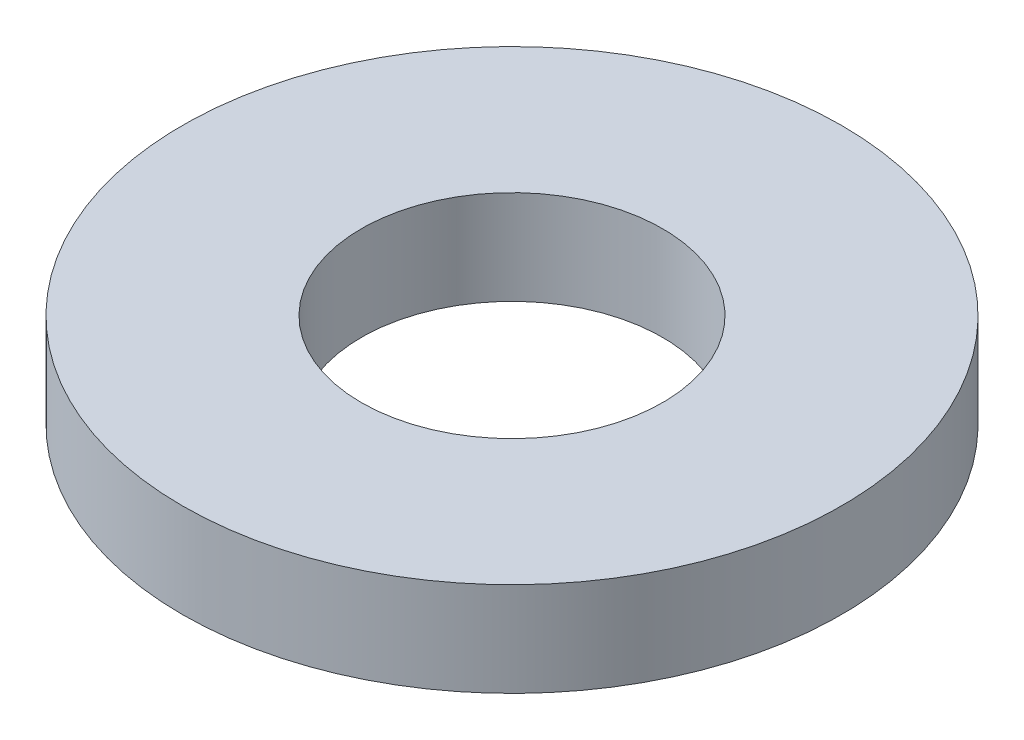
ISO-10303-21;
HEADER;
FILE_DESCRIPTION(('STEP AP214'),'2;1');
FILE_NAME('part.step','',(''),(''),'','','');
FILE_SCHEMA(('AUTOMOTIVE_DESIGN { 1 0 10303 214 1 1 1 1 }'));
ENDSEC;
DATA;
#1=APPLICATION_CONTEXT('core data for automotive mechanical design processes');
#2=APPLICATION_PROTOCOL_DEFINITION('international standard','automotive_design',2000,#1);
#3=PRODUCT_CONTEXT('',#1,'mechanical');
#4=PRODUCT('Part','Part','',(#3));
#5=PRODUCT_RELATED_PRODUCT_CATEGORY('part','',(#4));
#6=PRODUCT_DEFINITION_FORMATION('','',#4);
#7=PRODUCT_DEFINITION_CONTEXT('part definition',#1,'design');
#8=PRODUCT_DEFINITION('design','',#6,#7);
#9=PRODUCT_DEFINITION_SHAPE('','',#8);
#10=(LENGTH_UNIT() NAMED_UNIT(*) SI_UNIT(.MILLI.,.METRE.));
#11=(NAMED_UNIT(*) PLANE_ANGLE_UNIT() SI_UNIT($,.RADIAN.));
#12=(NAMED_UNIT(*) SI_UNIT($,.STERADIAN.) SOLID_ANGLE_UNIT());
#13=UNCERTAINTY_MEASURE_WITH_UNIT(LENGTH_MEASURE(1.E-05),#10,'distance_accuracy_value','');
#14=(GEOMETRIC_REPRESENTATION_CONTEXT(3) GLOBAL_UNCERTAINTY_ASSIGNED_CONTEXT((#13)) GLOBAL_UNIT_ASSIGNED_CONTEXT((#10,
#11,#12)) REPRESENTATION_CONTEXT('',''));
#15=CARTESIAN_POINT('',(0.,0.,0.));
#16=DIRECTION('',(0.,0.,1.));
#17=DIRECTION('',(1.,0.,0.));
#18=AXIS2_PLACEMENT_3D('',#15,#16,#17);
#19=CARTESIAN_POINT('',(0.,2.5,0.));
#20=DIRECTION('',(0.,1.,0.));
#21=DIRECTION('',(0.,0.,1.));
#22=AXIS2_PLACEMENT_3D('',#19,#20,#21);
#23=PLANE('',#22);
#24=CARTESIAN_POINT('',(0.,2.5,0.));
#25=DIRECTION('',(0.,1.,0.));
#26=DIRECTION('',(0.,0.,1.));
#27=AXIS2_PLACEMENT_3D('',#24,#25,#26);
#28=CIRCLE('',#27,17.5);
#29=CARTESIAN_POINT('',(0.,2.5,17.5));
#30=VERTEX_POINT('',#29);
#31=EDGE_CURVE('E10',#30,#30,#28,.T.);
#32=ORIENTED_EDGE('',*,*,#31,.T.);
#33=EDGE_LOOP('',(#32));
#34=FACE_BOUND('',#33,.T.);
#35=CARTESIAN_POINT('',(0.,2.5,0.));
#36=DIRECTION('',(0.,1.,0.));
#37=DIRECTION('',(0.,0.,1.));
#38=AXIS2_PLACEMENT_3D('',#35,#36,#37);
#39=CIRCLE('',#38,8.);
#40=CARTESIAN_POINT('',(0.,2.5,8.));
#41=VERTEX_POINT('',#40);
#42=EDGE_CURVE('E48',#41,#41,#39,.T.);
#43=ORIENTED_EDGE('',*,*,#42,.F.);
#44=EDGE_LOOP('',(#43));
#45=FACE_BOUND('',#44,.T.);
#46=ADVANCED_FACE('F40',(#34,#45),#23,.T.);
#47=CARTESIAN_POINT('',(0.,-2.5,0.));
#48=DIRECTION('',(0.,1.,0.));
#49=DIRECTION('',(0.,0.,1.));
#50=AXIS2_PLACEMENT_3D('',#47,#48,#49);
#51=PLANE('',#50);
#52=CARTESIAN_POINT('',(0.,-2.5,0.));
#53=DIRECTION('',(0.,1.,0.));
#54=DIRECTION('',(0.,0.,1.));
#55=AXIS2_PLACEMENT_3D('',#52,#53,#54);
#56=CIRCLE('',#55,17.5);
#57=CARTESIAN_POINT('',(0.,-2.5,17.5));
#58=VERTEX_POINT('',#57);
#59=EDGE_CURVE('E41',#58,#58,#56,.T.);
#60=ORIENTED_EDGE('',*,*,#59,.F.);
#61=EDGE_LOOP('',(#60));
#62=FACE_BOUND('',#61,.T.);
#63=CARTESIAN_POINT('',(0.,-2.5,0.));
#64=DIRECTION('',(0.,1.,0.));
#65=DIRECTION('',(0.,0.,1.));
#66=AXIS2_PLACEMENT_3D('',#63,#64,#65);
#67=CIRCLE('',#66,8.);
#68=CARTESIAN_POINT('',(0.,-2.5,8.));
#69=VERTEX_POINT('',#68);
#70=EDGE_CURVE('E49',#69,#69,#67,.T.);
#71=ORIENTED_EDGE('',*,*,#70,.T.);
#72=EDGE_LOOP('',(#71));
#73=FACE_BOUND('',#72,.T.);
#74=ADVANCED_FACE('F58',(#62,#73),#51,.F.);
#75=CARTESIAN_POINT('',(0.,2.5,0.));
#76=DIRECTION('',(0.,-1.,0.));
#77=DIRECTION('',(0.,0.,-1.));
#78=AXIS2_PLACEMENT_3D('',#75,#76,#77);
#79=CYLINDRICAL_SURFACE('',#78,17.5);
#80=ORIENTED_EDGE('',*,*,#31,.F.);
#81=EDGE_LOOP('',(#80));
#82=FACE_BOUND('',#81,.T.);
#83=ORIENTED_EDGE('',*,*,#59,.T.);
#84=EDGE_LOOP('',(#83));
#85=FACE_BOUND('',#84,.T.);
#86=ADVANCED_FACE('F39',(#82,#85),#79,.T.);
#87=CARTESIAN_POINT('',(0.,2.5,0.));
#88=DIRECTION('',(0.,-1.,0.));
#89=DIRECTION('',(0.,0.,-1.));
#90=AXIS2_PLACEMENT_3D('',#87,#88,#89);
#91=CYLINDRICAL_SURFACE('',#90,8.);
#92=ORIENTED_EDGE('',*,*,#42,.T.);
#93=EDGE_LOOP('',(#92));
#94=FACE_BOUND('',#93,.T.);
#95=ORIENTED_EDGE('',*,*,#70,.F.);
#96=EDGE_LOOP('',(#95));
#97=FACE_BOUND('',#96,.T.);
#98=ADVANCED_FACE('F57',(#94,#97),#91,.F.);
#99=CLOSED_SHELL('',(#46,#74,#86,#98));
#100=MANIFOLD_SOLID_BREP('B2',#99);
#101=ADVANCED_BREP_SHAPE_REPRESENTATION('',(#18,#100),#14);
#102=SHAPE_DEFINITION_REPRESENTATION(#9,#101);
ENDSEC;
END-ISO-10303-21;
